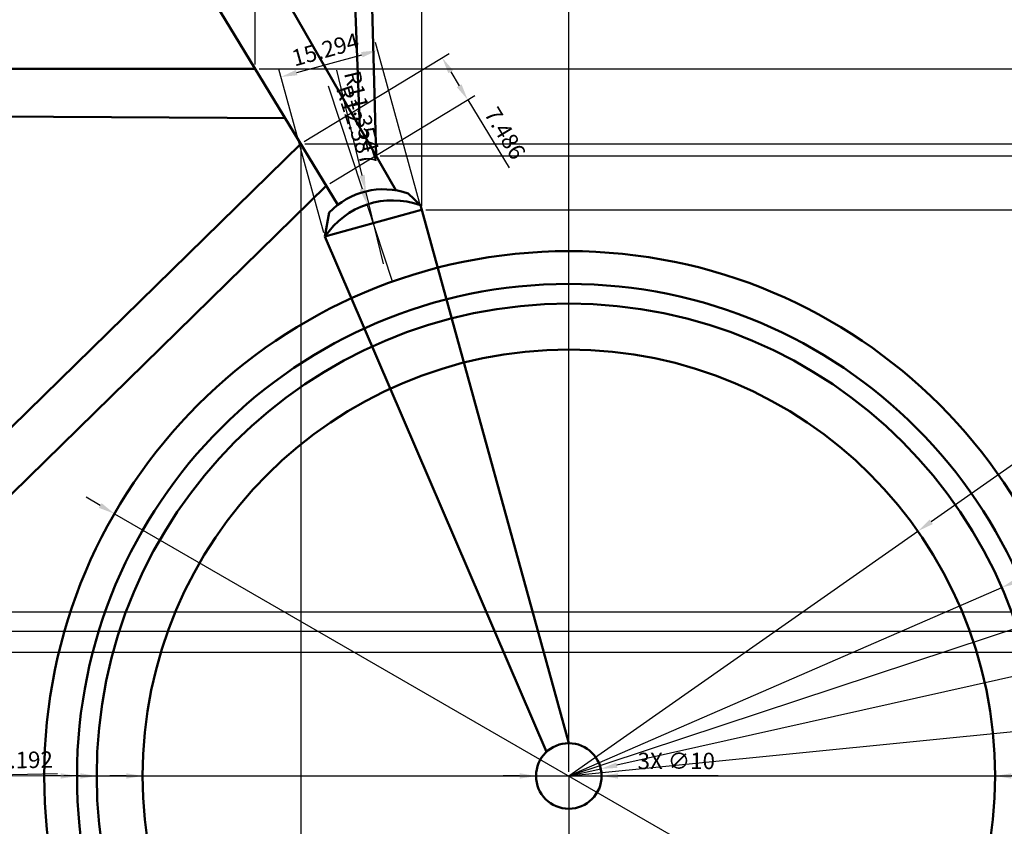
# Model space of a CAD drawing. Units: millimetres. Extents: x 1068 to 1546, y 1743 to 2032.
# Tile 7 of 9: x 1318 to 1469, y 1842 to 1965. Entities that reach past the tile are written whole.
import ezdxf

# ---------------------------------------------------------------- set-up
doc = ezdxf.new("R2010")
doc.units = ezdxf.units.MM
for name, color, linetype, lineweight in [('M-CONS', 8, 'Continuous', 18), ('M-DIMS', 2, 'Continuous', 25), ('M-OUTL', 7, 'Continuous', 50)]:
    doc.layers.add(name, color=color, linetype=linetype, lineweight=lineweight)
doc.styles.get("Standard").update_dxf_attribs({"font": 'arial.ttf'})
doc.dimstyles.new('ISO-25', dxfattribs={"dimtxt": 2.5, "dimasz": 2.5, "dimexe": 1.25, "dimexo": 0.625, "dimtad": 1, "dimtxsty": 'Standard', "dimcen": 2.5, "dimadec": 0, "dimazin": 0, "dimtfac": 1, "dimtmove": 0, "dimatfit": 3, "dimfxl": 1, "dimarcsym": 0})

# ---------------------------------------------------------------- blocks, each defined once
blk = doc.blocks.new('*D5')
at = {"layer": 'Defpoints', "color": 0, "transparency": 16777216}
for p in [(1177.23, 1849.76), (1402.23, 1849.76), (1402.23, 1747.98)]:
    blk.add_point(p, dxfattribs=at)
at = {"layer": 'M-DIMS', "color": 0, "lineweight": -2, "transparency": 16777216}
for p, q in [((1177.23, 1849.14), (1177.23, 1746.73)), ((1402.23, 1849.14), (1402.23, 1746.73)), ((1179.73, 1747.98), (1399.73, 1747.98))]:
    blk.add_line(p, q, dxfattribs=at)
at = {"layer": 'M-DIMS', "color": 0, "transparency": 16777216}
for points in [[(1179.73, 1748.39), (1179.73, 1747.56), (1177.23, 1747.98)], [(1399.73, 1748.39), (1399.73, 1747.56), (1402.23, 1747.98)]]:
    blk.add_solid(points, dxfattribs=at)
at = {"layer": 'M-DIMS', "color": 0, "transparency": 16777216, "insert": (1289.73, 1749.88), "char_height": 2.5, "attachment_point": 5}
blk.add_mtext('225', dxfattribs=at)
blk = doc.blocks.new('*D7')
at = {"layer": 'Defpoints', "color": 0, "transparency": 16777216}
for p in [(1407.11, 1850.85), (1402.23, 1849.76)]:
    blk.add_point(p, dxfattribs=at)
at = {"layer": 'M-DIMS', "color": 0, "lineweight": -2, "transparency": 16777216}
for p, q in [((1545.85, 1881.92), (1409.55, 1851.4)), ((1402.23, 1849.76), (1407.11, 1850.85))]:
    blk.add_line(p, q, dxfattribs=at)
at = {"layer": 'M-DIMS', "color": 0, "transparency": 16777216}
blk.add_solid([(1409.46, 1851.81), (1409.64, 1850.99), (1407.11, 1850.85)], dxfattribs=at)
at = {"layer": 'M-DIMS', "color": 0, "transparency": 16777216, "insert": (1542.85, 1883.19), "char_height": 2.5, "attachment_point": 5, "rotation": 12.6193}
blk.add_mtext('R5', dxfattribs=at)
blk = doc.blocks.new('*D8')
at = {"layer": 'Defpoints', "color": 0, "transparency": 16777216}
for p in [(1455.46, 1887.07), (1402.23, 1849.76)]:
    blk.add_point(p, dxfattribs=at)
at = {"layer": 'M-DIMS', "color": 0, "lineweight": -2, "transparency": 16777216}
for p, q in [((1514.78, 1928.64), (1457.51, 1888.5)), ((1402.23, 1849.76), (1455.46, 1887.07))]:
    blk.add_line(p, q, dxfattribs=at)
at = {"layer": 'M-DIMS', "color": 0, "transparency": 16777216}
blk.add_solid([(1457.27, 1888.84), (1457.75, 1888.16), (1455.46, 1887.07)], dxfattribs=at)
at = {"layer": 'M-DIMS', "color": 0, "transparency": 16777216, "insert": (1510.72, 1928.11), "char_height": 2.5, "attachment_point": 5, "rotation": 35.0221}
blk.add_mtext('R65', dxfattribs=at)
blk = doc.blocks.new('*D9')
at = {"layer": 'Defpoints', "color": 0, "transparency": 16777216}
for p in [(1468.25, 1878.49), (1402.23, 1849.76)]:
    blk.add_point(p, dxfattribs=at)
at = {"layer": 'M-DIMS', "color": 0, "lineweight": -2, "transparency": 16777216}
for p, q in [((1521.25, 1901.55), (1470.54, 1879.49)), ((1402.23, 1849.76), (1468.25, 1878.49))]:
    blk.add_line(p, q, dxfattribs=at)
at = {"layer": 'M-DIMS', "color": 0, "transparency": 16777216}
blk.add_solid([(1470.38, 1879.87), (1470.71, 1879.1), (1468.25, 1878.49)], dxfattribs=at)
at = {"layer": 'M-DIMS', "color": 0, "transparency": 16777216, "insert": (1517.2, 1901.84), "char_height": 2.5, "attachment_point": 5, "rotation": 23.5148}
blk.add_mtext('R72', dxfattribs=at)
blk = doc.blocks.new('*D10')
at = {"layer": 'Defpoints', "color": 0, "transparency": 16777216}
for p in [(1473.44, 1873.29), (1402.23, 1849.76)]:
    blk.add_point(p, dxfattribs=at)
at = {"layer": 'M-DIMS', "color": 0, "lineweight": -2, "transparency": 16777216}
for p, q in [((1525.61, 1890.52), (1475.82, 1874.07)), ((1402.23, 1849.76), (1473.44, 1873.29))]:
    blk.add_line(p, q, dxfattribs=at)
at = {"layer": 'M-DIMS', "color": 0, "transparency": 16777216}
blk.add_solid([(1475.69, 1874.47), (1475.95, 1873.68), (1473.44, 1873.29)], dxfattribs=at)
at = {"layer": 'M-DIMS', "color": 0, "transparency": 16777216, "insert": (1521.57, 1891.19), "char_height": 2.5, "attachment_point": 5, "rotation": 18.2811}
blk.add_mtext('R75', dxfattribs=at)
blk = doc.blocks.new('*D11')
at = {"layer": 'Defpoints', "color": 0, "transparency": 16777216}
for p in [(1481.83, 1857.72), (1402.23, 1849.76)]:
    blk.add_point(p, dxfattribs=at)
at = {"layer": 'M-DIMS', "color": 0, "lineweight": -2, "transparency": 16777216}
for p, q in [((1537.65, 1863.3), (1484.32, 1857.97)), ((1402.23, 1849.76), (1481.83, 1857.72))]:
    blk.add_line(p, q, dxfattribs=at)
at = {"layer": 'M-DIMS', "color": 0, "transparency": 16777216}
blk.add_solid([(1484.28, 1858.38), (1484.36, 1857.56), (1481.83, 1857.72)], dxfattribs=at)
at = {"layer": 'M-DIMS', "color": 0, "transparency": 16777216, "insert": (1533.87, 1864.83), "char_height": 2.5, "attachment_point": 5, "rotation": 5.7095}
blk.add_mtext('R80', dxfattribs=at)
blk = doc.blocks.new('*D22')
at = {"layer": 'Defpoints', "color": 0, "transparency": 16777216}
for p in [(1354.41, 2023.87), (1212.56, 1957.56), (1354.41, 1957.56)]:
    blk.add_point(p, dxfattribs=at)
at = {"layer": 'M-DIMS', "color": 0, "lineweight": -2, "transparency": 16777216}
for p, q in [((1212.56, 1958.19), (1212.56, 2025.12)), ((1354.41, 1958.19), (1354.41, 2025.12)), ((1215.06, 2023.87), (1351.91, 2023.87))]:
    blk.add_line(p, q, dxfattribs=at)
at = {"layer": 'M-DIMS', "color": 0, "transparency": 16777216}
for points in [[(1215.06, 2024.29), (1215.06, 2023.46), (1212.56, 2023.87)], [(1351.91, 2024.29), (1351.91, 2023.46), (1354.41, 2023.87)]]:
    blk.add_solid(points, dxfattribs=at)
at = {"layer": 'M-DIMS', "color": 0, "transparency": 16777216, "insert": (1283.48, 2026), "char_height": 2.5, "attachment_point": 5}
blk.add_mtext('141,85', dxfattribs=at)
blk = doc.blocks.new('*D24')
at = {"layer": 'Defpoints', "color": 0, "transparency": 16777216}
for p in [(1270.79, 1850.31), (1402.23, 1850.31), (1402.23, 1761.81)]:
    blk.add_point(p, dxfattribs=at)
at = {"layer": 'M-DIMS', "color": 0, "lineweight": -2, "transparency": 16777216}
for p, q in [((1270.79, 1849.68), (1270.79, 1760.56)), ((1402.23, 1849.68), (1402.23, 1760.56)), ((1273.29, 1761.81), (1399.73, 1761.81))]:
    blk.add_line(p, q, dxfattribs=at)
at = {"layer": 'M-DIMS', "color": 0, "transparency": 16777216}
for points in [[(1273.29, 1762.23), (1273.29, 1761.4), (1270.79, 1761.81)], [(1399.73, 1762.23), (1399.73, 1761.4), (1402.23, 1761.81)]]:
    blk.add_solid(points, dxfattribs=at)
at = {"layer": 'M-DIMS', "color": 0, "transparency": 16777216, "insert": (1336.51, 1763.94), "char_height": 2.5, "attachment_point": 5}
blk.add_mtext('131,44', dxfattribs=at)
blk = doc.blocks.new('*D25')
at = {"layer": 'Defpoints', "color": 0, "transparency": 16777216}
for p in [(1376.21, 2002.95), (1507.48, 2002.95), (1402.23, 1769.76)]:
    blk.add_point(p, dxfattribs=at)
at = {"layer": 'M-DIMS', "color": 0, "lineweight": -2, "transparency": 16777216}
for p, q in [((1376.84, 2002.95), (1508.73, 2002.95)), ((1507.48, 1772.26), (1507.48, 2000.45)), ((1402.85, 1769.76), (1508.73, 1769.76))]:
    blk.add_line(p, q, dxfattribs=at)
at = {"layer": 'M-DIMS', "color": 0, "transparency": 16777216}
for points in [[(1507.06, 2000.45), (1507.89, 2000.45), (1507.48, 2002.95)], [(1507.06, 1772.26), (1507.89, 1772.26), (1507.48, 1769.76)]]:
    blk.add_solid(points, dxfattribs=at)
at = {"layer": 'M-DIMS', "color": 0, "transparency": 16777216, "insert": (1505.58, 1886.35), "char_height": 2.5, "attachment_point": 5, "rotation": 90}
blk.add_mtext('233.2', dxfattribs=at)
blk = doc.blocks.new('*D27')
at = {"layer": 'Defpoints', "color": 0, "transparency": 16777216}
for p in [(1270.79, 1874.76), (1507.48, 1874.76), (1272.28, 1871.84)]:
    blk.add_point(p, dxfattribs=at)
at = {"layer": 'M-DIMS', "color": 0, "lineweight": -2, "transparency": 16777216}
for p, q in [((1507.48, 1877.26), (1507.48, 1887.52)), ((1271.41, 1874.76), (1508.73, 1874.76)), ((1507.48, 1871.84), (1507.48, 1874.76)), ((1272.9, 1871.84), (1508.73, 1871.84)), ((1507.48, 1869.34), (1507.48, 1866.84))]:
    blk.add_line(p, q, dxfattribs=at)
at = {"layer": 'M-DIMS', "color": 0, "transparency": 16777216}
for points in [[(1507.06, 1877.26), (1507.89, 1877.26), (1507.48, 1874.76)], [(1507.06, 1869.34), (1507.89, 1869.34), (1507.48, 1871.84)]]:
    blk.add_solid(points, dxfattribs=at)
at = {"layer": 'M-DIMS', "color": 0, "transparency": 16777216, "insert": (1505.58, 1883.64), "char_height": 2.5, "attachment_point": 5, "rotation": 90}
blk.add_mtext('2.92', dxfattribs=at)
blk = doc.blocks.new('*D34')
at = {"layer": 'Defpoints', "color": 0, "transparency": 16777216}
for p in [(1379.79, 1936.04), (1507.48, 1936.04), (1402.23, 1849.76)]:
    blk.add_point(p, dxfattribs=at)
at = {"layer": 'M-DIMS', "color": 0, "lineweight": -2, "transparency": 16777216}
for p, q in [((1380.41, 1936.04), (1508.73, 1936.04)), ((1507.48, 1852.26), (1507.48, 1933.54)), ((1402.85, 1849.76), (1508.73, 1849.76))]:
    blk.add_line(p, q, dxfattribs=at)
at = {"layer": 'M-DIMS', "color": 0, "transparency": 16777216}
for points in [[(1507.06, 1933.54), (1507.89, 1933.54), (1507.48, 1936.04)], [(1507.06, 1852.26), (1507.89, 1852.26), (1507.48, 1849.76)]]:
    blk.add_solid(points, dxfattribs=at)
at = {"layer": 'M-DIMS', "color": 0, "transparency": 16777216, "insert": (1505.58, 1892.9), "char_height": 2.5, "attachment_point": 5, "rotation": 90}
blk.add_mtext('86.28', dxfattribs=at)
blk = doc.blocks.new('*D35')
at = {"layer": 'Defpoints', "color": 0, "transparency": 16777216}
for p in [(1354.41, 1957.56), (1507.48, 1957.56), (1379.79, 1936.04)]:
    blk.add_point(p, dxfattribs=at)
at = {"layer": 'M-DIMS', "color": 0, "lineweight": -2, "transparency": 16777216}
for p, q in [((1355.03, 1957.56), (1508.73, 1957.56)), ((1507.48, 1938.54), (1507.48, 1955.06)), ((1380.41, 1936.04), (1508.73, 1936.04))]:
    blk.add_line(p, q, dxfattribs=at)
at = {"layer": 'M-DIMS', "color": 0, "transparency": 16777216}
for points in [[(1507.06, 1955.06), (1507.89, 1955.06), (1507.48, 1957.56)], [(1507.06, 1938.54), (1507.89, 1938.54), (1507.48, 1936.04)]]:
    blk.add_solid(points, dxfattribs=at)
at = {"layer": 'M-DIMS', "color": 0, "transparency": 16777216, "insert": (1505.58, 1946.8), "char_height": 2.5, "attachment_point": 5, "rotation": 90}
blk.add_mtext('21.52', dxfattribs=at)
blk = doc.blocks.new('*D36')
at = {"layer": 'Defpoints', "color": 0, "transparency": 16777216}
for p in [(1346.59, 1989.88), (1507.48, 1989.88), (1354.41, 1957.56)]:
    blk.add_point(p, dxfattribs=at)
at = {"layer": 'M-DIMS', "color": 0, "lineweight": -2, "transparency": 16777216}
for p, q in [((1347.22, 1989.88), (1508.73, 1989.88)), ((1507.48, 1960.06), (1507.48, 1987.38)), ((1355.03, 1957.56), (1508.73, 1957.56))]:
    blk.add_line(p, q, dxfattribs=at)
at = {"layer": 'M-DIMS', "color": 0, "transparency": 16777216}
for points in [[(1507.06, 1987.38), (1507.89, 1987.38), (1507.48, 1989.88)], [(1507.06, 1960.06), (1507.89, 1960.06), (1507.48, 1957.56)]]:
    blk.add_solid(points, dxfattribs=at)
at = {"layer": 'M-DIMS', "color": 0, "transparency": 16777216, "insert": (1505.58, 1973.72), "char_height": 2.5, "attachment_point": 5, "rotation": 90}
blk.add_mtext('32.32', dxfattribs=at)
blk = doc.blocks.new('*D39')
at = {"layer": 'Defpoints', "color": 0, "transparency": 16777216}
for p in [(1379.79, 2028.2), (1355.9, 1999.79), (1379.79, 1936.04)]:
    blk.add_point(p, dxfattribs=at)
at = {"layer": 'M-DIMS', "color": 0, "lineweight": -2, "transparency": 16777216}
for p, q in [((1355.9, 2000.41), (1355.9, 2029.45)), ((1379.79, 1936.66), (1379.79, 2029.45)), ((1358.4, 2028.2), (1377.29, 2028.2))]:
    blk.add_line(p, q, dxfattribs=at)
at = {"layer": 'M-DIMS', "color": 0, "transparency": 16777216}
for points in [[(1358.4, 2028.61), (1358.4, 2027.78), (1355.9, 2028.2)], [(1377.29, 2028.61), (1377.29, 2027.78), (1379.79, 2028.2)]]:
    blk.add_solid(points, dxfattribs=at)
at = {"layer": 'M-DIMS', "color": 0, "transparency": 16777216, "insert": (1367.84, 2030.1), "char_height": 2.5, "attachment_point": 5}
blk.add_mtext('23.89', dxfattribs=at)
blk = doc.blocks.new('*D40')
at = {"layer": 'Defpoints', "color": 0, "transparency": 16777216}
for p in [(1402.23, 2028.2), (1379.79, 1936.04), (1402.23, 1849.76)]:
    blk.add_point(p, dxfattribs=at)
at = {"layer": 'M-DIMS', "color": 0, "lineweight": -2, "transparency": 16777216}
for p, q in [((1379.79, 1936.66), (1379.79, 2029.45)), ((1402.23, 1850.39), (1402.23, 2029.45)), ((1382.29, 2028.2), (1399.73, 2028.2))]:
    blk.add_line(p, q, dxfattribs=at)
at = {"layer": 'M-DIMS', "color": 0, "transparency": 16777216}
for points in [[(1382.29, 2028.61), (1382.29, 2027.78), (1379.79, 2028.2)], [(1399.73, 2028.61), (1399.73, 2027.78), (1402.23, 2028.2)]]:
    blk.add_solid(points, dxfattribs=at)
at = {"layer": 'M-DIMS', "color": 0, "transparency": 16777216, "insert": (1391.01, 2030.08), "char_height": 2.5, "attachment_point": 5}
blk.add_mtext('22.44', dxfattribs=at)
blk = doc.blocks.new('*D43')
at = {"layer": 'Defpoints', "color": 0, "transparency": 16777216}
for p in [(1373.07, 1960.38), (1379.79, 1936.04), (1365.04, 1931.97)]:
    blk.add_point(p, dxfattribs=at)
at = {"layer": 'M-DIMS', "color": 0, "lineweight": -2, "transparency": 16777216}
for p, q in [((1379.62, 1936.64), (1372.73, 1961.58)), ((1360.73, 1956.97), (1370.66, 1959.71)), ((1364.88, 1932.57), (1357.99, 1957.51))]:
    blk.add_line(p, q, dxfattribs=at)
at = {"layer": 'M-DIMS', "color": 0, "transparency": 16777216}
for points in [[(1370.55, 1960.11), (1370.77, 1959.31), (1373.07, 1960.38)], [(1360.62, 1957.38), (1360.84, 1956.57), (1358.32, 1956.31)]]:
    blk.add_solid(points, dxfattribs=at)
at = {"layer": 'M-DIMS', "color": 0, "transparency": 16777216, "insert": (1365.19, 1960.18), "char_height": 2.5, "attachment_point": 5, "rotation": 15.4356}
blk.add_mtext('15.294', dxfattribs=at)
blk = doc.blocks.new('*D47')
at = {"layer": 'Defpoints', "color": 0, "transparency": 16777216}
for p in [(1361.34, 1946.14), (1282.2, 1868.65), (1361.34, 1744.51)]:
    blk.add_point(p, dxfattribs=at)
at = {"layer": 'M-DIMS', "color": 0, "lineweight": -2, "transparency": 16777216}
for p, q in [((1361.34, 1945.51), (1361.34, 1743.26)), ((1282.2, 1868.03), (1282.2, 1743.26)), ((1284.7, 1744.51), (1358.84, 1744.51))]:
    blk.add_line(p, q, dxfattribs=at)
at = {"layer": 'M-DIMS', "color": 0, "transparency": 16777216}
for points in [[(1284.7, 1744.93), (1284.7, 1744.1), (1282.2, 1744.51)], [(1358.84, 1744.93), (1358.84, 1744.1), (1361.34, 1744.51)]]:
    blk.add_solid(points, dxfattribs=at)
at = {"layer": 'M-DIMS', "color": 0, "transparency": 16777216, "insert": (1321.77, 1746.41), "char_height": 2.5, "attachment_point": 5}
blk.add_mtext('79.14', dxfattribs=at)
blk = doc.blocks.new('*D48')
at = {"layer": 'Defpoints', "color": 0, "transparency": 16777216}
for p in [(1361.34, 1946.14), (1507.48, 1946.14), (1282.2, 1868.65)]:
    blk.add_point(p, dxfattribs=at)
at = {"layer": 'M-DIMS', "color": 0, "lineweight": -2, "transparency": 16777216}
for p, q in [((1361.96, 1946.14), (1508.73, 1946.14)), ((1507.48, 1871.15), (1507.48, 1943.64)), ((1282.82, 1868.65), (1508.73, 1868.65))]:
    blk.add_line(p, q, dxfattribs=at)
at = {"layer": 'M-DIMS', "color": 0, "transparency": 16777216}
for points in [[(1507.06, 1943.64), (1507.89, 1943.64), (1507.48, 1946.14)], [(1507.06, 1871.15), (1507.89, 1871.15), (1507.48, 1868.65)]]:
    blk.add_solid(points, dxfattribs=at)
at = {"layer": 'M-DIMS', "color": 0, "transparency": 16777216, "insert": (1505.58, 1907.39), "char_height": 2.5, "attachment_point": 5, "rotation": 90}
blk.add_mtext('77.49', dxfattribs=at)
blk = doc.blocks.new('*D49')
at = {"layer": 'Defpoints', "color": 0, "transparency": 16777216}
for p in [(1386.81, 1952.84), (1361.34, 1946.14), (1365.22, 1939.74)]:
    blk.add_point(p, dxfattribs=at)
at = {"layer": 'M-DIMS', "color": 0, "lineweight": -2, "transparency": 16777216}
for p, q in [((1361.87, 1946.46), (1383.99, 1959.89)), ((1384.22, 1957.1), (1385.51, 1954.98)), ((1365.76, 1940.06), (1387.88, 1953.49)), ((1386.81, 1952.84), (1393.12, 1942.44))]:
    blk.add_line(p, q, dxfattribs=at)
at = {"layer": 'M-DIMS', "color": 0, "transparency": 16777216}
for points in [[(1384.58, 1957.32), (1383.86, 1956.89), (1382.92, 1959.24)], [(1385.87, 1955.19), (1385.15, 1954.76), (1386.81, 1952.84)]]:
    blk.add_solid(points, dxfattribs=at)
at = {"layer": 'M-DIMS', "color": 0, "transparency": 16777216, "insert": (1392.24, 1947.56), "char_height": 2.5, "attachment_point": 5, "rotation": 301.2584}
blk.add_mtext('7.486', dxfattribs=at)
blk = doc.blocks.new('*D51')
at = {"layer": 'Defpoints', "color": 0, "transparency": 16777216}
for p in [(1402.23, 2028.2), (1390.93, 1989.88), (1402.23, 1849.76)]:
    blk.add_point(p, dxfattribs=at)
at = {"layer": 'M-DIMS', "color": 0, "lineweight": -2, "transparency": 16777216}
for p, q in [((1390.93, 1990.51), (1390.93, 2029.45)), ((1402.23, 1850.39), (1402.23, 2029.45)), ((1393.43, 2028.2), (1399.73, 2028.2)), ((1402.23, 2028.2), (1416.12, 2028.2))]:
    blk.add_line(p, q, dxfattribs=at)
at = {"layer": 'M-DIMS', "color": 0, "transparency": 16777216}
for points in [[(1393.43, 2028.61), (1393.43, 2027.78), (1390.93, 2028.2)], [(1399.73, 2028.61), (1399.73, 2027.78), (1402.23, 2028.2)]]:
    blk.add_solid(points, dxfattribs=at)
at = {"layer": 'M-DIMS', "color": 0, "transparency": 16777216, "insert": (1410.42, 2030.1), "char_height": 2.5, "attachment_point": 5}
blk.add_mtext('11.296', dxfattribs=at)
blk = doc.blocks.new('*D52')
at = {"layer": 'Defpoints', "color": 0, "transparency": 16777216}
for p in [(1372.84, 1944.27), (1402.23, 1849.76), (1507.48, 1849.76)]:
    blk.add_point(p, dxfattribs=at)
at = {"layer": 'M-DIMS', "color": 0, "lineweight": -2, "transparency": 16777216}
for p, q in [((1373.47, 1944.27), (1508.73, 1944.27)), ((1507.48, 1941.77), (1507.48, 1852.26)), ((1402.85, 1849.76), (1508.73, 1849.76))]:
    blk.add_line(p, q, dxfattribs=at)
at = {"layer": 'M-DIMS', "color": 0, "transparency": 16777216}
for points in [[(1507.06, 1941.77), (1507.89, 1941.77), (1507.48, 1944.27)], [(1507.06, 1852.26), (1507.89, 1852.26), (1507.48, 1849.76)]]:
    blk.add_solid(points, dxfattribs=at)
at = {"layer": 'M-DIMS', "color": 0, "transparency": 16777216, "insert": (1505.58, 1897.02), "char_height": 2.5, "attachment_point": 5, "rotation": 90}
blk.add_mtext('94.51', dxfattribs=at)
blk = doc.blocks.new('*D53')
at = {"layer": 'Defpoints', "color": 0, "transparency": 16777216}
for p in [(1332.93, 1889.74), (1471.52, 1809.79)]:
    blk.add_point(p, dxfattribs=at)
at = {"layer": 'M-DIMS', "color": 0, "lineweight": -2, "transparency": 16777216}
for p, q in [((1330.77, 1890.99), (1328.6, 1892.24)), ((1332.93, 1889.74), (1471.52, 1809.79)), ((1517.21, 1783.43), (1473.69, 1808.54))]:
    blk.add_line(p, q, dxfattribs=at)
at = {"layer": 'M-DIMS', "color": 0, "transparency": 16777216}
for points in [[(1330.98, 1891.35), (1330.56, 1890.63), (1332.93, 1889.74)], [(1473.9, 1808.9), (1473.48, 1808.18), (1471.52, 1809.79)]]:
    blk.add_solid(points, dxfattribs=at)
at = {"layer": 'M-DIMS', "color": 0, "transparency": 16777216, "insert": (1514.09, 1787.51), "char_height": 2.5, "attachment_point": 5, "rotation": 330.0197}
blk.add_mtext('∅160', dxfattribs=at)
blk = doc.blocks.new('*D54')
at = {"layer": 'Defpoints', "color": 0, "transparency": 16777216}
for p in [(1327.23, 1849.76), (1477.23, 1849.76)]:
    blk.add_point(p, dxfattribs=at)
at = {"layer": 'M-DIMS', "color": 0, "lineweight": -2, "transparency": 16777216}
for p, q in [((1324.73, 1849.76), (1322.23, 1849.76)), ((1327.23, 1849.76), (1477.23, 1849.76)), ((1526.97, 1849.76), (1479.73, 1849.76))]:
    blk.add_line(p, q, dxfattribs=at)
at = {"layer": 'M-DIMS', "color": 0, "transparency": 16777216}
for points in [[(1324.73, 1850.18), (1324.73, 1849.35), (1327.23, 1849.76)], [(1479.73, 1850.18), (1479.73, 1849.35), (1477.23, 1849.76)]]:
    blk.add_solid(points, dxfattribs=at)
at = {"layer": 'M-DIMS', "color": 0, "transparency": 16777216, "insert": (1522.23, 1851.73), "char_height": 2.5, "attachment_point": 5, "rotation": 359.9998}
blk.add_mtext('∅150', dxfattribs=at)
blk = doc.blocks.new('*D55')
at = {"layer": 'Defpoints', "color": 0, "transparency": 16777216}
for p in [(1330.23, 1849.76), (1474.23, 1849.76)]:
    blk.add_point(p, dxfattribs=at)
at = {"layer": 'M-DIMS', "color": 0, "lineweight": -2, "transparency": 16777216}
for p, q in [((1327.73, 1849.76), (1325.23, 1849.76)), ((1330.23, 1849.76), (1474.23, 1849.76)), ((1522.17, 1849.76), (1476.73, 1849.76))]:
    blk.add_line(p, q, dxfattribs=at)
at = {"layer": 'M-DIMS', "color": 0, "transparency": 16777216}
for points in [[(1327.73, 1850.18), (1327.73, 1849.35), (1330.23, 1849.76)], [(1476.73, 1850.18), (1476.73, 1849.35), (1474.23, 1849.76)]]:
    blk.add_solid(points, dxfattribs=at)
at = {"layer": 'M-DIMS', "color": 0, "transparency": 16777216, "insert": (1517.43, 1851.73), "char_height": 2.5, "attachment_point": 5, "rotation": 359.9997}
blk.add_mtext('∅144', dxfattribs=at)
blk = doc.blocks.new('*D56')
at = {"layer": 'Defpoints', "color": 0, "transparency": 16777216}
for p in [(1337.23, 1849.76), (1467.23, 1849.76)]:
    blk.add_point(p, dxfattribs=at)
at = {"layer": 'M-DIMS', "color": 0, "lineweight": -2, "transparency": 16777216}
for p, q in [((1334.73, 1849.76), (1332.23, 1849.76)), ((1337.23, 1849.76), (1467.23, 1849.76)), ((1513.61, 1849.76), (1469.73, 1849.76))]:
    blk.add_line(p, q, dxfattribs=at)
at = {"layer": 'M-DIMS', "color": 0, "transparency": 16777216}
for points in [[(1334.73, 1850.18), (1334.73, 1849.35), (1337.23, 1849.76)], [(1469.73, 1850.18), (1469.73, 1849.35), (1467.23, 1849.76)]]:
    blk.add_solid(points, dxfattribs=at)
at = {"layer": 'M-DIMS', "color": 0, "transparency": 16777216, "insert": (1506.23, 1851.73), "char_height": 2.5, "attachment_point": 5, "rotation": 359.9997}
blk.add_mtext('2X ∅130', dxfattribs=at)
blk = doc.blocks.new('*D61')
at = {"layer": 'Defpoints', "color": 0, "transparency": 16777216}
for p in [(1397.23, 1849.76), (1407.23, 1849.76)]:
    blk.add_point(p, dxfattribs=at)
at = {"layer": 'M-DIMS', "color": 0, "lineweight": -2, "transparency": 16777216}
for p, q in [((1394.73, 1849.76), (1392.23, 1849.76)), ((1397.23, 1849.76), (1407.23, 1849.76)), ((1425.01, 1849.76), (1409.73, 1849.76))]:
    blk.add_line(p, q, dxfattribs=at)
at = {"layer": 'M-DIMS', "color": 0, "transparency": 16777216}
for points in [[(1394.73, 1850.18), (1394.73, 1849.35), (1397.23, 1849.76)], [(1409.73, 1850.18), (1409.73, 1849.35), (1407.23, 1849.76)]]:
    blk.add_solid(points, dxfattribs=at)
at = {"layer": 'M-DIMS', "color": 0, "transparency": 16777216, "insert": (1418.62, 1851.73), "char_height": 2.5, "attachment_point": 5, "rotation": 359.9963}
blk.add_mtext('3X ∅10', dxfattribs=at)
blk = doc.blocks.new('*D69')
at = {"layer": 'Defpoints', "color": 0, "transparency": 16777216}
for p in [(1371.49, 1936.88), (1375.36, 1925.12)]:
    blk.add_point(p, dxfattribs=at)
at = {"layer": 'M-DIMS', "color": 0, "lineweight": -2, "transparency": 16777216}
for p, q in [((1365.53, 1954.95), (1370.7, 1939.26)), ((1375.36, 1925.12), (1371.49, 1936.88))]:
    blk.add_line(p, q, dxfattribs=at)
at = {"layer": 'M-DIMS', "color": 0, "transparency": 16777216}
blk.add_solid([(1371.1, 1939.39), (1370.31, 1939.13), (1371.49, 1936.88)], dxfattribs=at)
at = {"layer": 'M-DIMS', "color": 0, "transparency": 16777216, "insert": (1369.53, 1948.88), "char_height": 2.5, "attachment_point": 5, "rotation": 288.2428}
blk.add_mtext('R12.387', dxfattribs=at)
blk = doc.blocks.new('*D70')
at = {"layer": 'Defpoints', "color": 0, "transparency": 16777216}
for p in [(1371.28, 1938.88), (1373.95, 1927.84)]:
    blk.add_point(p, dxfattribs=at)
at = {"layer": 'M-DIMS', "color": 0, "lineweight": -2, "transparency": 16777216}
for p, q in [((1366.82, 1957.36), (1370.69, 1941.31)), ((1373.95, 1927.84), (1371.28, 1938.88))]:
    blk.add_line(p, q, dxfattribs=at)
at = {"layer": 'M-DIMS', "color": 0, "transparency": 16777216}
blk.add_solid([(1371.1, 1941.41), (1370.29, 1941.21), (1371.28, 1938.88)], dxfattribs=at)
at = {"layer": 'M-DIMS', "color": 0, "transparency": 16777216, "insert": (1370.31, 1950.99), "char_height": 2.5, "attachment_point": 5, "rotation": 283.5799}
blk.add_mtext('R11.354', dxfattribs=at)
blk = doc.blocks.new('*D85')
at = {"layer": 'Defpoints', "color": 0, "transparency": 16777216}
for p in [(1304.02, 1849.7), (1307.22, 1849.76)]:
    blk.add_point(p, dxfattribs=at)
at = {"layer": 'M-DIMS', "color": 0, "lineweight": -2, "transparency": 16777216}
for p, q in [((1324.27, 1850.07), (1309.71, 1849.81)), ((1304.02, 1849.7), (1307.22, 1849.76))]:
    blk.add_line(p, q, dxfattribs=at)
at = {"layer": 'M-DIMS', "color": 0, "transparency": 16777216}
blk.add_solid([(1309.71, 1850.22), (1309.72, 1849.39), (1307.22, 1849.76)], dxfattribs=at)
at = {"layer": 'M-DIMS', "color": 0, "transparency": 16777216, "insert": (1318.21, 1851.86), "char_height": 2.5, "attachment_point": 5, "rotation": 1.0509}
blk.add_mtext('R3.192', dxfattribs=at)

msp = doc.modelspace()

# ---------------------------------------------------------------- linework, layer by layer
at = {"layer": 'M-CONS'}
msp.add_line((1172.2281, 1849.7623), (1402.2281, 1849.7623), dxfattribs=at)
at = {"layer": 'M-OUTL'}
for p, q in [((1346.5904, 1989.8822), (1375.8591, 1939.0334)), ((1368.9422, 1985.2737), (1370.3848, 1948.5438)), ((1371.687, 1986.2339), (1372.8438, 1944.2719)), ((1366.9956, 1936.8189), (1338.924, 1983.0643)), ((1212.5594, 1957.5607), (1352.9598, 1957.5607)), ((1352.9598, 1957.5607), (1354.405, 1957.5607)), ((1216.7245, 1950.8999), (1358.9799, 1950.024)), ((1282.1954, 1868.6519), (1361.339, 1946.1377)), ((1288.8124, 1864.9272), (1365.2237, 1939.738)), ((1379.5868, 1936.7621), (1377.7269, 1938.5478)), ((1365.0442, 1931.9687), (1379.7864, 1936.0393)), ((1365.0442, 1931.9687), (1365.6972, 1935.6425)), ((1402.2281, 1854.7623), (1379.5868, 1936.7621)), ((1398.8448, 1853.4437), (1365.0442, 1931.9687))]:
    msp.add_line(p, q, dxfattribs=at)
for radius in [80, 75, 72, 65, 5]:
    msp.add_circle((1402.2281, 1849.7623), radius, dxfattribs=at)
for centre, radius, start, end in [((1373.9468, 1927.842), 11.3535, 70.552306, 136.603057), ((1375.3638, 1925.1172), 12.387, 70.066762, 146.418526)]:
    msp.add_arc(centre, radius, start, end, dxfattribs=at)

# ---------------------------------------------------------------- dimensions: what is measured, and where the dimension line sits
at = {"layer": 'M-DIMS'}
for base, p1, p2, override, picture, middle in [((1379.7864, 2028.1976), (1355.8981, 1999.7899), (1379.7864, 1936.0393), {"dimdec": 2, "dimlfac": 1, "dimrnd": 0, "dimzin": 0, "dimdsep": 46, "dimlunit": 2}, '*D39', (1367.8422, 2030.0999)), ((1402.2281, 2028.1976), (1379.7864, 1936.0393), (1402.2281, 1849.7623), {"dimdec": 2, "dimlfac": 1, "dimrnd": 0, "dimzin": 0, "dimdsep": 46, "dimlunit": 2}, '*D40', (1391.0073, 2030.0777)), ((1402.2281, 2028.1976), (1390.9319, 1989.8822), (1402.2281, 1849.7623), {"dimdec": 3, "dimlfac": 1, "dimrnd": 0, "dimzin": 0, "dimdsep": 46, "dimlunit": 2}, '*D51', (1410.4239, 2030.099)), ((1354.405, 2023.8738), (1212.5594, 1957.5607), (1354.405, 1957.5607), {"dimclrd": 0, "dimclre": 0, "dimclrt": 0}, '*D22', (1283.4822, 2026.0012)), ((1361.339, 1744.5123), (1282.1954, 1868.6519), (1361.339, 1946.1377), {"dimdec": 2, "dimlfac": 1, "dimrnd": 0, "dimzin": 0, "dimdsep": 46, "dimlunit": 2}, '*D47', (1321.7672, 1746.4138)), ((1402.2281, 1761.8125), (1270.787, 1850.3085), (1402.2281, 1850.3085), {"dimclrd": 0, "dimclre": 0, "dimclrt": 0}, '*D24', (1336.5076, 1763.9399)), ((1402.2281, 1747.9766), (1177.2281, 1849.7623), (1402.2281, 1849.7623), {"dimclrd": 0, "dimclre": 0, "dimclrt": 0}, '*D5', (1289.7281, 1749.8781))]:
    dim = msp.add_linear_dim(base=base, p1=p1, p2=p2, dimstyle='ISO-25', override=override, dxfattribs=at)
    dim.commit()
    dim.dimension.update_dxf_attribs({"geometry": picture, "text_midpoint": middle})
for base, p1, p2, angle, override, picture, middle in [((1507.4781, 2002.9476), (1402.2281, 1769.7623), (1376.2106, 2002.9476), 90, {"dimdec": 1, "dimlfac": 1, "dimrnd": 0, "dimzin": 0, "dimdsep": 46, "dimlunit": 2}, '*D25', (1505.5758, 1886.355)), ((1507.4781, 1989.8822), (1354.405, 1957.5607), (1346.5904, 1989.8822), 90, {"dimdec": 2, "dimlfac": 1, "dimrnd": 0, "dimzin": 0, "dimdsep": 46, "dimlunit": 2}, '*D36', (1505.5758, 1973.7215)), ((1373.066, 1960.3785), (1365.0442, 1931.9687), (1379.7864, 1936.0393), 15.435581, {"dimdec": 3, "dimlfac": 1, "dimrnd": 0, "dimzin": 0, "dimdsep": 46, "dimlunit": 2}, '*D43', (1365.1888, 1960.1761)), ((1386.8083, 1952.8402), (1361.339, 1946.1377), (1365.2237, 1939.738), 301.258412, {"dimdec": 3, "dimlfac": 1, "dimrnd": 0, "dimzin": 0, "dimdsep": 46, "dimlunit": 2}, '*D49', (1392.2383, 1947.5591)), ((1507.4781, 1957.5607), (1379.7864, 1936.0393), (1354.405, 1957.5607), 90, {"dimdec": 2, "dimlfac": 1, "dimrnd": 0, "dimzin": 0, "dimdsep": 46, "dimlunit": 2}, '*D35', (1505.5767, 1946.8)), ((1507.4781, 1946.1377), (1282.1954, 1868.6519), (1361.339, 1946.1377), 90, {"dimdec": 2, "dimlfac": 1, "dimrnd": 0, "dimzin": 0, "dimdsep": 46, "dimlunit": 2}, '*D48', (1505.5767, 1907.3948)), ((1507.4781, 1849.7623), (1372.8438, 1944.2719), (1402.2281, 1849.7623), 90, {"dimdec": 2, "dimlfac": 1, "dimrnd": 0, "dimzin": 0, "dimdsep": 46, "dimlunit": 2}, '*D52', (1505.5767, 1897.0171)), ((1507.4781, 1936.0393), (1402.2281, 1849.7623), (1379.7864, 1936.0393), 90, {"dimdec": 2, "dimlfac": 1, "dimrnd": 0, "dimzin": 0, "dimdsep": 46, "dimlunit": 2}, '*D34', (1505.5767, 1892.9008)), ((1507.4781, 1874.7623), (1272.2751, 1871.8409), (1270.787, 1874.7623), 90, {"dimdec": 2, "dimlfac": 1, "dimrnd": 0, "dimzin": 0, "dimdsep": 46, "dimlunit": 2}, '*D27', (1505.5767, 1883.6428))]:
    dim = msp.add_linear_dim(base=base, p1=p1, p2=p2, angle=angle, dimstyle='ISO-25', override=override, dxfattribs=at)
    dim.commit()
    dim.dimension.update_dxf_attribs({"geometry": picture, "text_midpoint": middle})
for center, mpoint, picture, middle in [((1373.9468, 1927.842), (1371.281, 1938.8781), '*D70', (1370.3112, 1950.9946)), ((1375.3638, 1925.1172), (1371.4861, 1936.8816), '*D69', (1369.533, 1948.884)), ((1304.0238, 1849.7019), (1307.2154, 1849.7604), '*D85', (1318.2052, 1851.8647))]:
    dim = msp.add_radius_dim(center=center, mpoint=mpoint, dimstyle='ISO-25', override={"dimdec": 3, "dimlfac": 1, "dimrnd": 0, "dimzin": 0, "dimdsep": 46, "dimlunit": 2}, dxfattribs=at)
    dim.commit()
    dim.dimension.update_dxf_attribs({"geometry": picture, "text_midpoint": middle})
for mpoint, picture, middle in [((1455.4586, 1887.0653), '*D8', (1511.8133, 1926.5577)), ((1468.249, 1878.4894), '*D9', (1517.9503, 1900.1154)), ((1473.4428, 1873.2883), '*D10', (1522.1694, 1889.3852)), ((1407.1073, 1850.8547), '*D7', (1543.265, 1881.3376)), ((1481.8313, 1857.7211), '*D11', (1534.0596, 1862.943))]:
    dim = msp.add_radius_dim(center=(1402.2281, 1849.7623), mpoint=mpoint, dimstyle='ISO-25', override={"dimclrd": 0, "dimclre": 0, "dimclrt": 0}, dxfattribs=at)
    dim.commit()
    dim.dimension.update_dxf_attribs({"geometry": picture, "text_midpoint": middle, "dimtype": 164})
for p1, p2, picture, middle in [((1332.9323, 1889.7385), (1471.5239, 1809.7862), '*D53', (1513.1014, 1785.8005)), ((1327.2281, 1849.7627), (1477.2281, 1849.762), '*D54', (1522.2281, 1849.7618)), ((1330.2281, 1849.7627), (1474.2281, 1849.762), '*D55', (1517.4281, 1849.7618))]:
    dim = msp.add_diameter_dim_2p(p1=p1, p2=p2, dimstyle='ISO-25', override={"dimdec": 0, "dimlfac": 1, "dimrnd": 0, "dimzin": 0, "dimdsep": 46, "dimlunit": 2}, dxfattribs=at)
    dim.commit()
    dim.dimension.update_dxf_attribs({"geometry": picture, "text_midpoint": middle, "dimtype": 163})
dim = msp.add_diameter_dim_2p(p1=(1337.2281, 1849.7627), p2=(1467.2281, 1849.762), text='2X <>', dimstyle='ISO-25', override={"dimdec": 0, "dimlfac": 1, "dimrnd": 0, "dimzin": 0, "dimdsep": 46, "dimlunit": 2}, dxfattribs=at)
dim.commit()
dim.dimension.update_dxf_attribs({"geometry": '*D56', "text_midpoint": (1506.2281, 1849.7618), "dimtype": 163})
dim = msp.add_diameter_dim_2p(p1=(1397.2281, 1849.7627), p2=(1407.2281, 1849.762), text='3X <>', dimstyle='ISO-25', override={"dimdec": 0, "dimlfac": 1, "dimrnd": 0, "dimzin": 0, "dimdsep": 46, "dimlunit": 2}, dxfattribs=at)
dim.commit()
dim.dimension.update_dxf_attribs({"geometry": '*D61', "text_midpoint": (1418.618, 1849.7613)})

doc.saveas('drawing.dxf')
